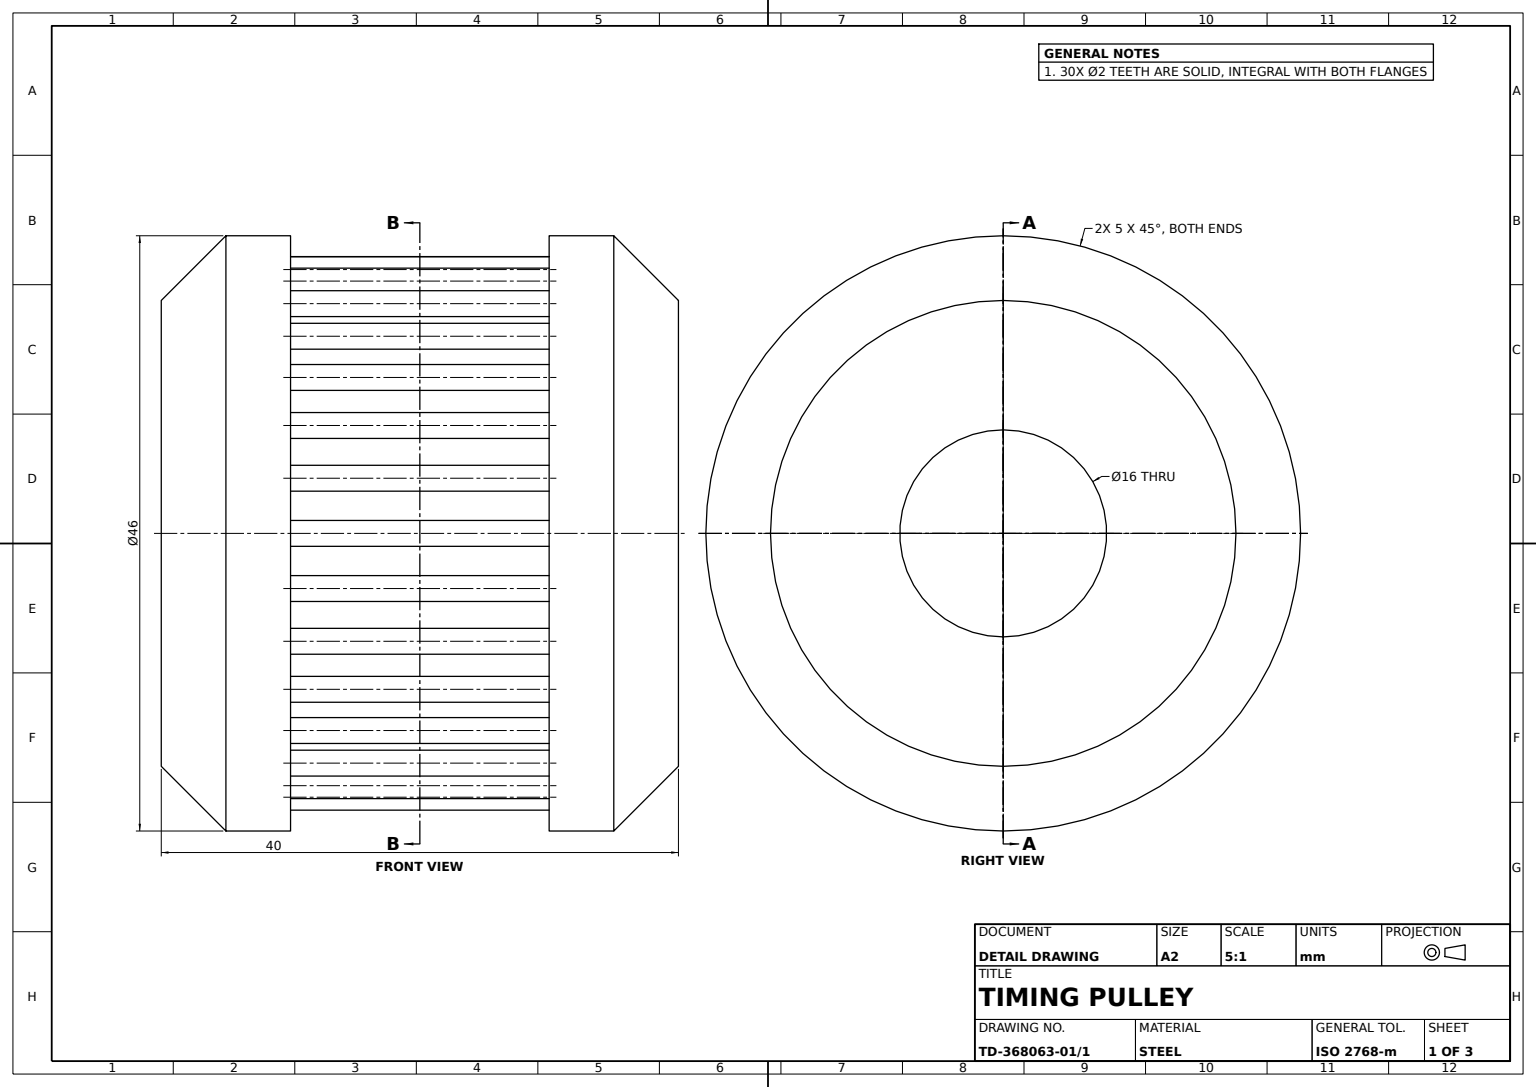
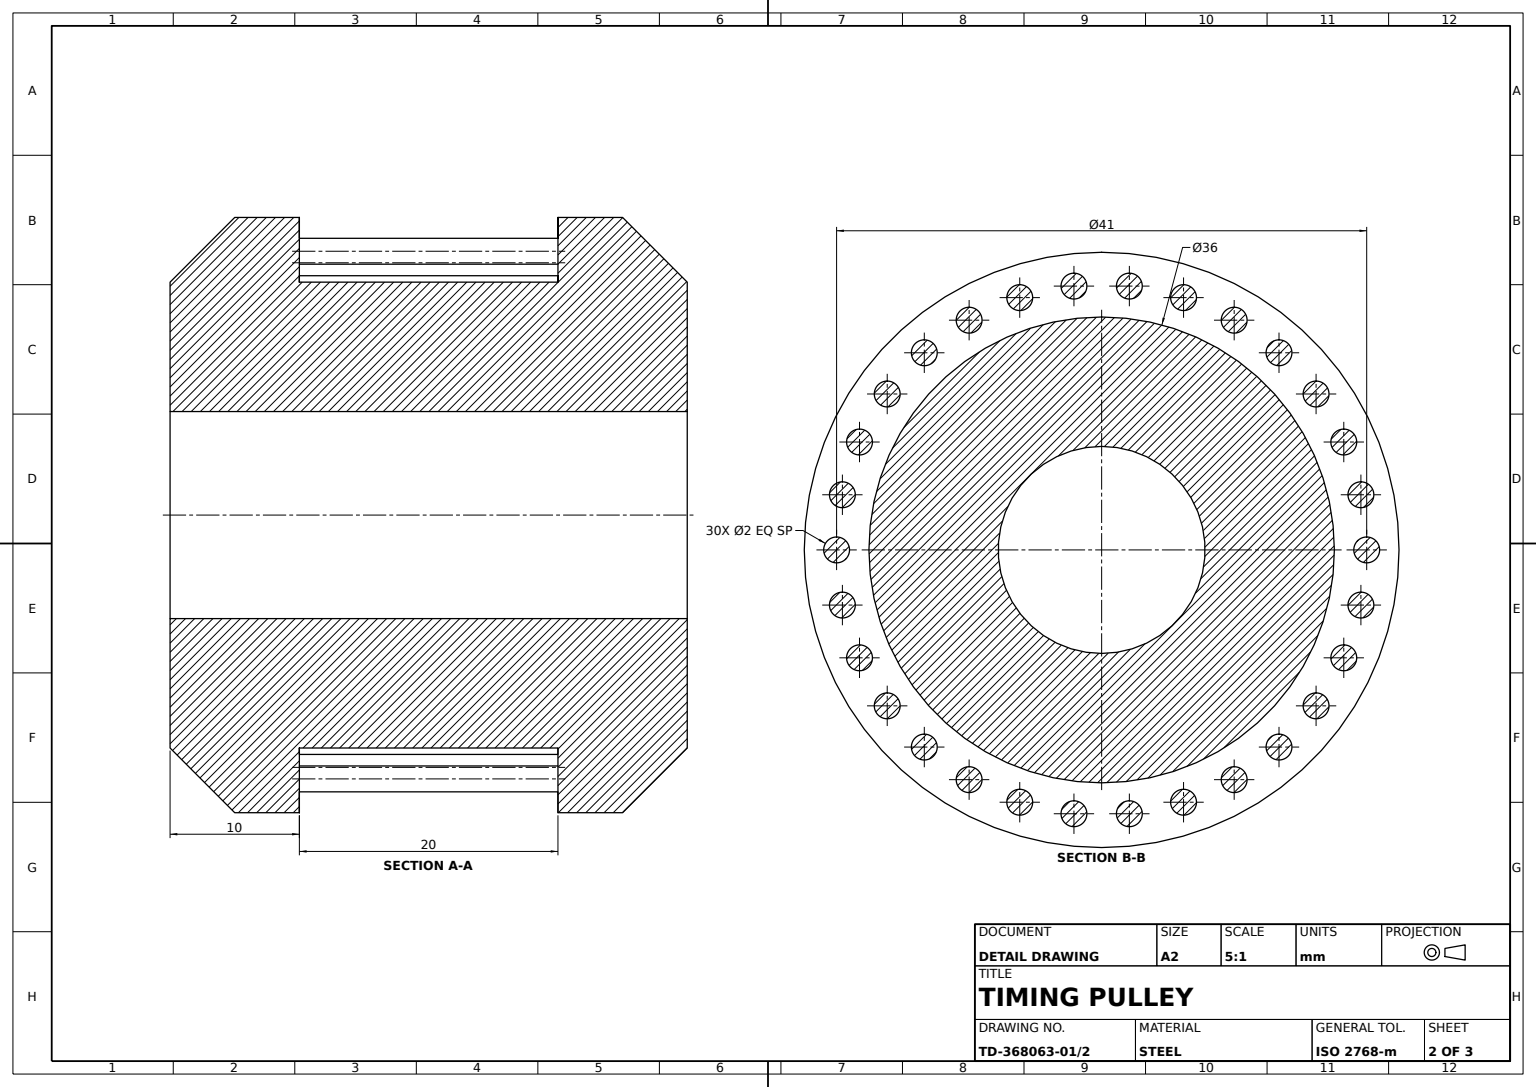
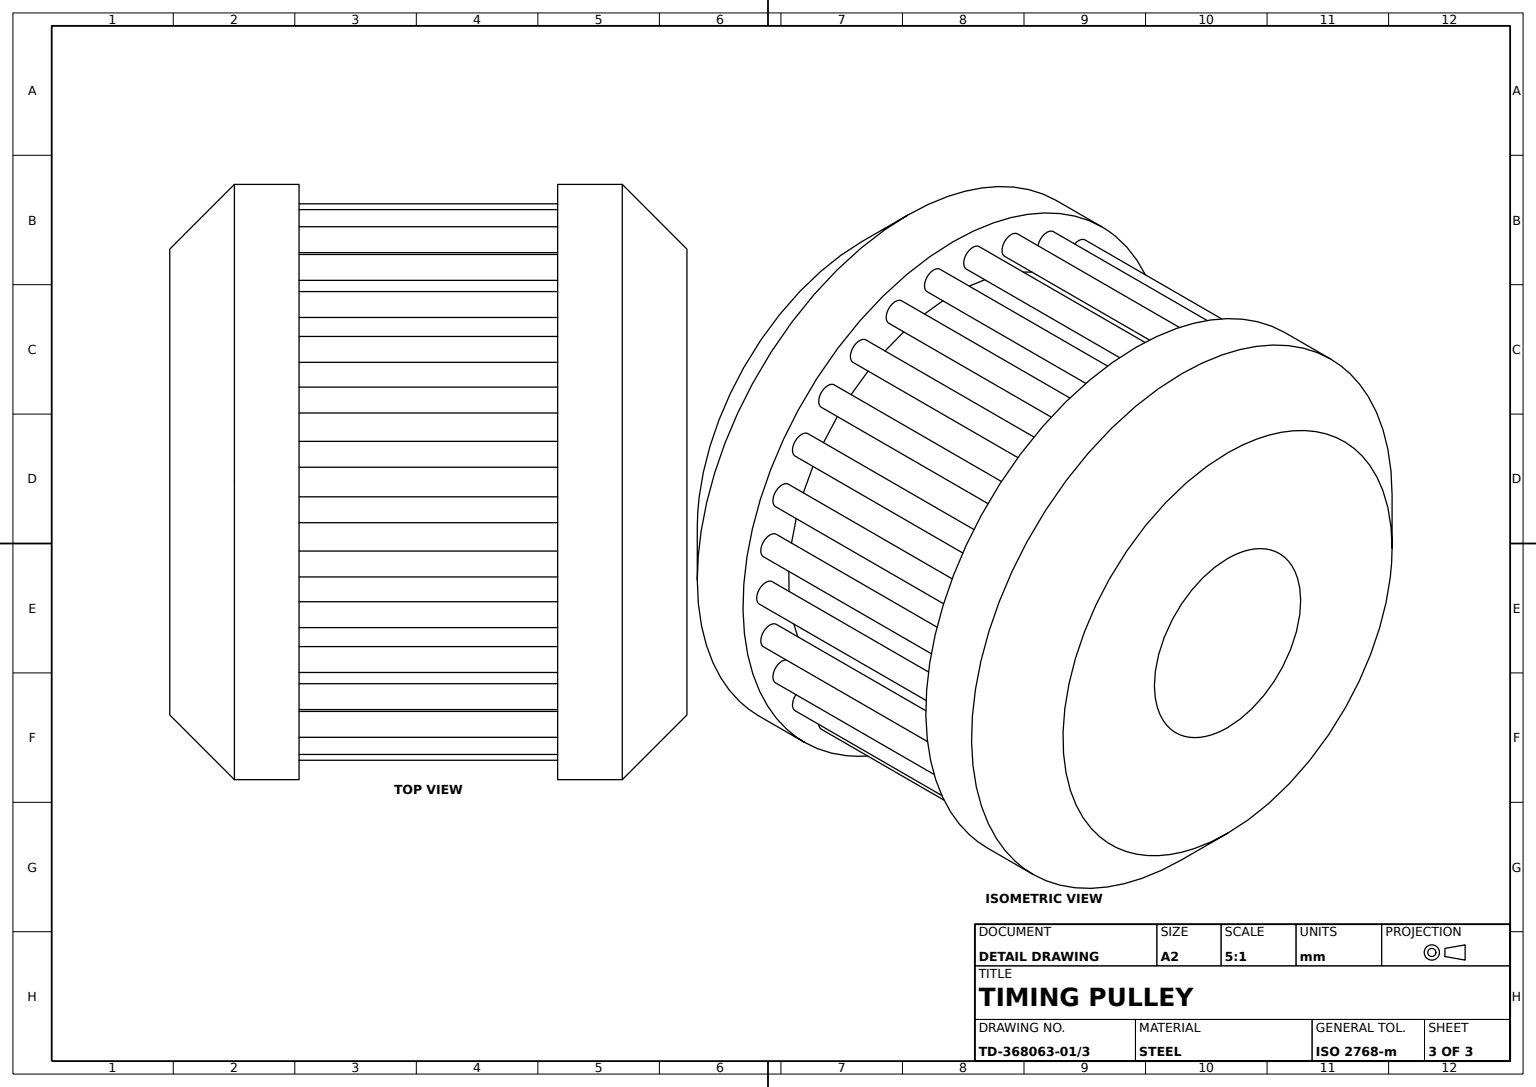
from build123d import *

# Parameters (mm, degrees)
TOOTH_PROFILE_R         = 1
TOOTH_DEPTH             = 20
TOOTH_PATTERN_30X_COUNT = 30


with BuildPart() as part:
    # Pulley Body Profile → Pulley Body (revolve)
    with BuildSketch(Plane.XY, mode=Mode.PRIVATE) as pulley_body_sk:
        Polygon((8, 40), (8, 0), (18, 0), (23, 5), (23, 10), (18, 10), (18, 30), (23, 30), (23, 35), (18, 40), align=None)
    revolve(pulley_body_sk.sketch.rotate(Axis((0, 32.636363636, 0), (0, -1, 0)), 180), axis=Axis((0, 32.636363636, 0), (0, -1, 0)))

    # Tooth Profile → Tooth (add)
    with BuildSketch(Plane.XZ.offset(-30)):
        with Locations(Location((0, 20.5, 0), (0, 0, 180))):
            Circle(TOOTH_PROFILE_R)
    tooth = extrude(amount=TOOTH_DEPTH)

    # Tooth Pattern 30x: Tooth ×30 about axis
    tooth_pattern_30x_axis = Axis((0, 0, 0), (0, 1, 0))
    for i in range(1, TOOTH_PATTERN_30X_COUNT):
        add(tooth.rotate(tooth_pattern_30x_axis, i * 360 / TOOTH_PATTERN_30X_COUNT))


solid = part.part
